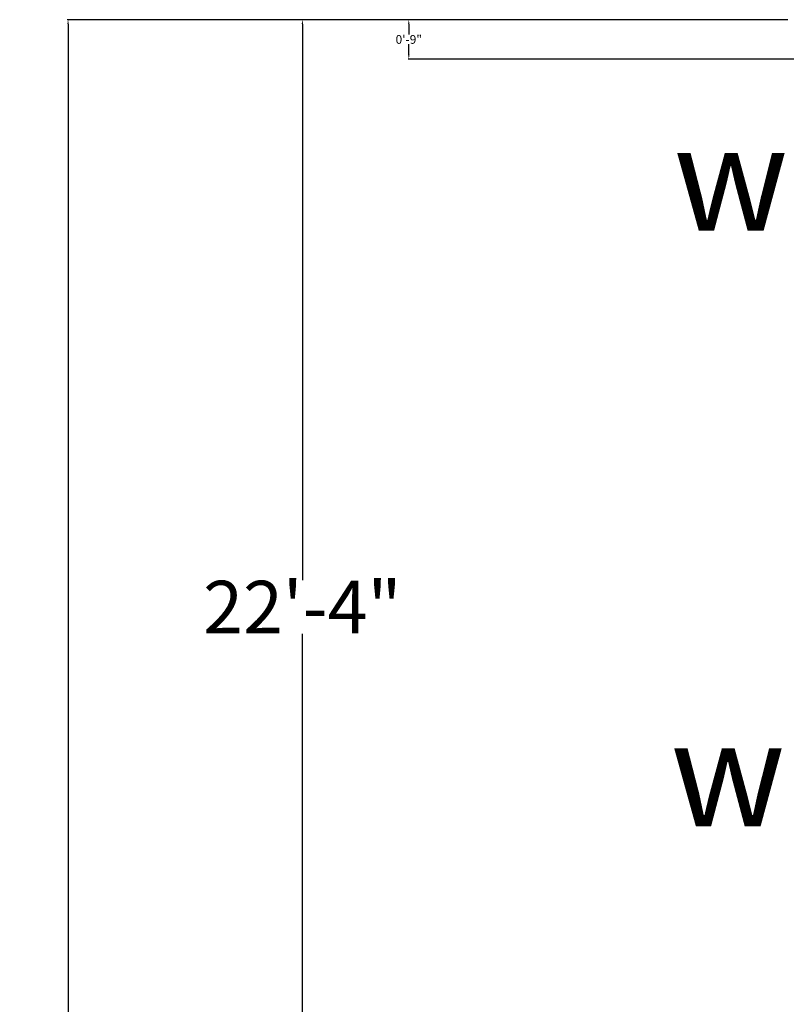
# Model space of a CAD drawing. Units: inches. Extents: x 409 to 7572, y 7 to 725.
# Tile 23 of 38: x 4151 to 4326, y 448 to 673. Entities that reach past the tile are written whole.
import ezdxf

# ---------------------------------------------------------------- set-up
doc = ezdxf.new("R2010")
doc.units = ezdxf.units.IN
doc.header["$MEASUREMENT"] = 0
doc.layers.add('A-ANNO-DIMS', color=2, linetype='Continuous', lineweight=18)
doc.layers.add('A-ANNO-SYMB', color=3, linetype='Continuous', lineweight=25)
doc.styles.get("Standard").update_dxf_attribs({"font": 'arial.ttf'})
doc.dimstyles.get("Standard").update_dxf_attribs({"dimtxt": 2, "dimasz": 1, "dimexe": 0.18, "dimexo": 0.0625, "dimgap": 0.09, "dimtad": 0, "dimtih": 1, "dimtoh": 1, "dimdec": 0, "dimzin": 0, "dimdsep": 46, "dimlunit": 3, "dimtxsty": 'Standard', "dimcen": 0.09, "dimadec": 0, "dimazin": 0, "dimtfac": 1, "dimtdec": 0, "dimtofl": 0, "dimtmove": 0, "dimatfit": 3, "dimfxl": 1, "dimtolj": 1, "dimtzin": 0, "dimarcsym": 0})

# ---------------------------------------------------------------- blocks, each defined once
blk = doc.blocks.new('*D104')
at = {"layer": 'A-ANNO-DIMS', "color": 0, "lineweight": -2, "transparency": 16777216}
for p, q in [((4325.88, 672.53), (4214.98, 672.53)), ((4215.16, 671.53), (4215.16, 544.65)), ((4215.16, 405.53), (4215.16, 532.42)), ((4325.88, 404.53), (4214.98, 404.53))]:
    blk.add_line(p, q, dxfattribs=at)
at = {"layer": 'A-ANNO-DIMS', "color": 0, "transparency": 16777216}
for points in [[(4214.99, 671.53), (4215.33, 671.53), (4215.16, 672.53)], [(4214.99, 405.53), (4215.33, 405.53), (4215.16, 404.53)]]:
    blk.add_solid(points, dxfattribs=at)
at = {"layer": 'DEFPOINTS', "color": 0, "transparency": 16777216}
for p in [(4325.94, 672.53), (4215.16, 404.53), (4325.94, 404.53)]:
    blk.add_point(p, dxfattribs=at)
at = {"layer": 'A-ANNO-DIMS', "color": 0, "transparency": 16777216, "insert": (4215.16, 538.53), "char_height": 2, "attachment_point": 5}
blk.add_mtext('\\A1;{\\H6x;22\'-4"}', dxfattribs=at)
blk = doc.blocks.new('*D93')
at = {"layer": 'A-ANNO-DIMS', "color": 0, "lineweight": -2, "transparency": 16777216}
for p, q in [((4325.88, 672.53), (4161.52, 672.53)), ((4161.7, 671.53), (4161.7, 420.75)), ((4161.7, 157.53), (4161.7, 408.31)), ((4325.88, 156.53), (4161.52, 156.53))]:
    blk.add_line(p, q, dxfattribs=at)
at = {"layer": 'A-ANNO-DIMS', "color": 0, "transparency": 16777216}
for points in [[(4161.54, 671.53), (4161.87, 671.53), (4161.7, 672.53)], [(4161.54, 157.53), (4161.87, 157.53), (4161.7, 156.53)]]:
    blk.add_solid(points, dxfattribs=at)
at = {"layer": 'DEFPOINTS', "color": 0, "transparency": 16777216}
for p in [(4325.94, 672.53), (4161.7, 156.53), (4325.94, 156.53)]:
    blk.add_point(p, dxfattribs=at)
at = {"layer": 'A-ANNO-DIMS', "color": 0, "transparency": 16777216, "insert": (4161.7, 414.53), "char_height": 2, "attachment_point": 5}
blk.add_mtext("\\A1;{\\H6x;43'}", dxfattribs=at)
blk = doc.blocks.new('*D188')
at = {"layer": 'A-ANNO-DIMS', "color": 0, "lineweight": -2, "transparency": 16777216}
for p, q in [((4325.88, 672.53), (4239.26, 672.53)), ((4239.44, 671.53), (4239.44, 669.14)), ((4239.44, 664.53), (4239.44, 666.92)), ((4334.88, 663.53), (4239.26, 663.53))]:
    blk.add_line(p, q, dxfattribs=at)
at = {"layer": 'A-ANNO-DIMS', "color": 0, "transparency": 16777216}
for points in [[(4239.27, 671.53), (4239.61, 671.53), (4239.44, 672.53)], [(4239.27, 664.53), (4239.61, 664.53), (4239.44, 663.53)]]:
    blk.add_solid(points, dxfattribs=at)
at = {"layer": 'DEFPOINTS', "color": 0, "transparency": 16777216}
for p in [(4325.94, 672.53), (4239.44, 663.53), (4334.94, 663.53)]:
    blk.add_point(p, dxfattribs=at)
at = {"layer": 'A-ANNO-DIMS', "color": 0, "transparency": 16777216, "insert": (4239.44, 668.03), "char_height": 2, "attachment_point": 5}
blk.add_mtext('\\A1;0\'-9"', dxfattribs=at)

msp = doc.modelspace()

# ---------------------------------------------------------------- texts
at = {"layer": 'A-ANNO-SYMB', "char_height": 24, "attachment_point": 1}
for insert in [(4299.79, 648.37), (4299.11, 512.53)]:
    msp.add_mtext_dynamic_manual_height_columns('w', width=18.2582, gutter_width=1, heights=[0], dxfattribs=dict(at, insert=insert))

# ---------------------------------------------------------------- dimensions: what is measured, and where the dimension line sits
at = {"layer": 'A-ANNO-DIMS'}
for base, p2, picture, middle in [((4161.7, 156.53), (4325.94, 156.53), '*D93', (4161.7, 414.53)), ((4215.16, 404.53), (4325.94, 404.53), '*D104', (4215.16, 538.53))]:
    dim = msp.add_linear_dim(base=base, p1=(4325.94, 672.53), p2=p2, angle=90, text='{\\H6x;<>}', dimstyle='Standard', override={"dimclrd": 0, "dimclre": 0, "dimclrt": 0}, dxfattribs=at)
    dim.commit()
    dim.dimension.update_dxf_attribs({"geometry": picture, "text_midpoint": middle})
dim = msp.add_linear_dim(base=(4239.44, 663.53), p1=(4325.94, 672.53), p2=(4334.94, 663.53), angle=90, dimstyle='Standard', override={"dimdec": 1, "dimlfac": 1, "dimrnd": 0, "dimzin": 1, "dimdsep": 46, "dimlunit": 4, "dimfrac": 2}, dxfattribs=at)
dim.commit()
dim.dimension.update_dxf_attribs({"geometry": '*D188', "text_midpoint": (4239.44, 668.03)})

doc.saveas('drawing.dxf')
